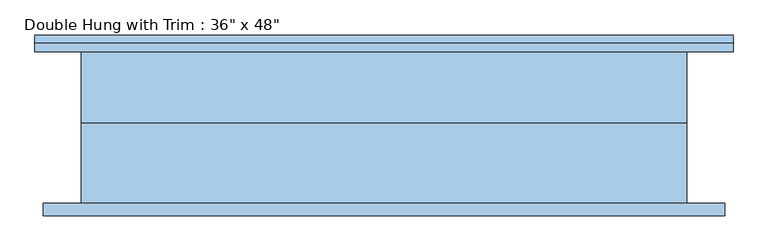
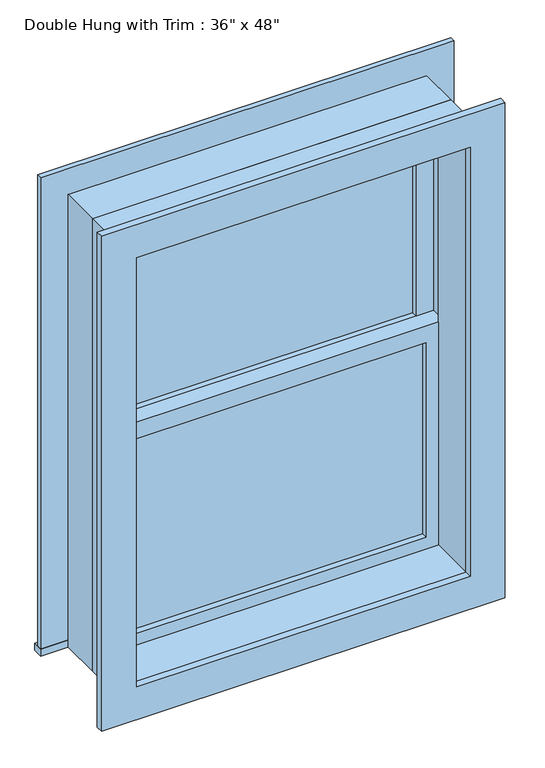
"""IFC4 building model written with IfcOpenShell, lengths in millimetres: window geometry."""

from ifc_helpers import new_model, si_unit, frame, origin, place, context, project, spatial, polyline, outline, extrude, source, transform, mapped, element, save


def window_f24a59ae(model_context):
    return source(origin(), model_context, "Body", "SweptSolid", [
        extrude(outline(polyline([(-393.7, 34.925), (393.7, 34.925), (393.7, 22.225), (-393.7, 22.225), (-393.7, 34.925)])), frame((0.0, 0.0, 977.9), z_axis=(0.0, 0.0, 1.0), x_axis=(1.0, 0.0, 0.0)), (0.0, 0.0, 1.0), 523.875),
        extrude(outline(polyline([(1546.225, -438.15), (933.45, -438.15), (933.45, 438.15), (1546.225, 438.15), (1546.225, -438.15)]), holes=[polyline([(1501.775, -393.7), (1501.775, 393.7), (977.9, 393.7), (977.9, -393.7), (1501.775, -393.7)])]), frame((0.0, 6.35, 0.0), z_axis=(0.0, 1.0, 0.0), x_axis=(0.0, 0.0, 1.0)), (0.0, 0.0, 1.0), 44.45),
        extrude(outline(polyline([(-527.05, 139.7), (527.05, 139.7), (527.05, 114.3), (-527.05, 114.3), (-527.05, 139.7)])), frame((0.0, 0.0, 914.4), z_axis=(0.0, 0.0, 1.0), x_axis=(1.0, 0.0, 0.0)), (0.0, 0.0, 1.0), 19.05),
        extrude(outline(polyline([(2114.55, -438.15), (2114.55, 438.15), (933.45, 438.15), (933.45, 527.05), (2203.45, 527.05), (2203.45, -527.05), (933.45, -527.05), (933.45, -438.15), (2114.55, -438.15)])), frame((0.0, 114.3, 0.0), z_axis=(0.0, 1.0, 0.0), x_axis=(0.0, 0.0, 1.0)), (0.0, 0.0, 1.0), 12.7),
        extrude(outline(polyline([(2190.75, 514.35), (2190.75, -514.35), (857.25, -514.35), (857.25, 514.35), (2190.75, 514.35)]), holes=[polyline([(2101.85, 425.45), (946.15, 425.45), (946.15, -425.45), (2101.85, -425.45), (2101.85, 425.45)])]), frame((0.0, -133.35, 0.0), z_axis=(0.0, 1.0, 0.0), x_axis=(0.0, 0.0, 1.0)), (0.0, 0.0, 1.0), 19.05),
        extrude(outline(polyline([(393.7, 66.675), (-393.7, 66.675), (-393.7, 79.375), (393.7, 79.375), (393.7, 66.675)])), frame((0.0, 0.0, 1546.225), z_axis=(0.0, 0.0, 1.0), x_axis=(1.0, 0.0, 0.0)), (0.0, 0.0, 1.0), 523.875),
        extrude(outline(polyline([(2114.55, -438.15), (1501.775, -438.15), (1501.775, 438.15), (2114.55, 438.15), (2114.55, -438.15)]), holes=[polyline([(2070.1, -393.7), (2070.1, 393.7), (1546.225, 393.7), (1546.225, -393.7), (2070.1, -393.7)])]), frame((0.0, 50.8, 0.0), z_axis=(0.0, 1.0, 0.0), x_axis=(0.0, 0.0, 1.0)), (0.0, 0.0, 1.0), 44.45),
        extrude(outline(polyline([(2133.6, -457.2), (914.4, -457.2), (914.4, 457.2), (2133.6, 457.2), (2133.6, -457.2)]), holes=[polyline([(2101.85, -425.45), (2101.85, 425.45), (946.15, 425.45), (946.15, -425.45), (2101.85, -425.45)])]), frame((0.0, -114.3, 0.0), z_axis=(0.0, 1.0, 0.0), x_axis=(0.0, 0.0, 1.0)), (0.0, 0.0, 1.0), 120.65),
        extrude(outline(polyline([(2133.6, 457.2), (2133.6, -457.2), (914.4, -457.2), (914.4, 457.2), (2133.6, 457.2)]), holes=[polyline([(2114.55, 438.15), (933.45, 438.15), (933.45, -438.15), (2114.55, -438.15), (2114.55, 438.15)])]), frame((0.0, 6.35, 0.0), z_axis=(0.0, 1.0, 0.0), x_axis=(0.0, 0.0, 1.0)), (0.0, 0.0, 1.0), 107.95),
    ])


if __name__ == "__main__":
    model = new_model("IFC4")
    model_context = context("Model", 3, world=origin())
    ifc_project = project(units=[si_unit("LENGTHUNIT", "METRE", prefix="MILLI")], contexts=[model_context])
    site = spatial("IfcSite", under=ifc_project)
    building = spatial("IfcBuilding", under=site)
    placement = place(None, origin())
    window_shape = window_f24a59ae(model_context)
    element("IfcWindow", 1, ObjectType="Double Hung with Trim : 36\" x 48\"", at=placement, inside=building, context=model_context, shape_type="MappedRepresentation", body=[
        mapped(window_shape, transform((0.0, 0.0, 0.0), x_axis=(1.0, 0.0, 0.0), y_axis=(0.0, 1.0, 0.0), z_axis=(0.0, 0.0, 1.0))),
    ])
    save(model, "model.ifc")

# Revit data of these elements
# Type "Double Hung with Trim : 36\" x 48\""
#   Type Mark = "10"
#   Construction Type Id = "GSP4R"
#   Assembly Code = "B2020100"
#   Analytic Construction = "1/8 in Pilkington single glazing"
#   Visual Light Transmittance = 0.9
#   Solar Heat Gain Coefficient = 0.78
#   Heat Transfer Coefficient (U) = 0.6496 BTU/(h·ft²·°F)
#   Height = 4' - 0"
#   Default Sill Height = 3' - 0"
#   Trim Projection - Ext. = 0' - 0 1/2"
#   Trim Projection - Int. = 0' - 0 3/4"
#   Trim Width - Exterior = 0' - 3 1/2"
#   Trim Width - Interior = 0' - 3 1/2"
#   Width = 3' - 0"
#   Window Inset = 0' - 0 3/4"
#   Define Thermal Properties by = 1
#   Glass Pane Material = Glass
#   Sash Material = Sash
#   Trim Exterior Material = Trim
#   Trim Interior Material = Trim
#   Wall Closure = (empty or 0)
# Element 1 (IfcWindow, "Double Hung with Trim : 36\" x 48\"")
#   Materials on its faces: "Sash", "Trim", "Glass"
# Materials
#   "Glass": class "Glass", colour RGB 0 128 192, transparency 0.75, Description = "Soda Lime Glass", Cost = 0
#   "Sash": class "Wood", colour RGB 224 178 126, transparency 0
#   "Trim": class "Wood", colour RGB 224 178 126, transparency 0
